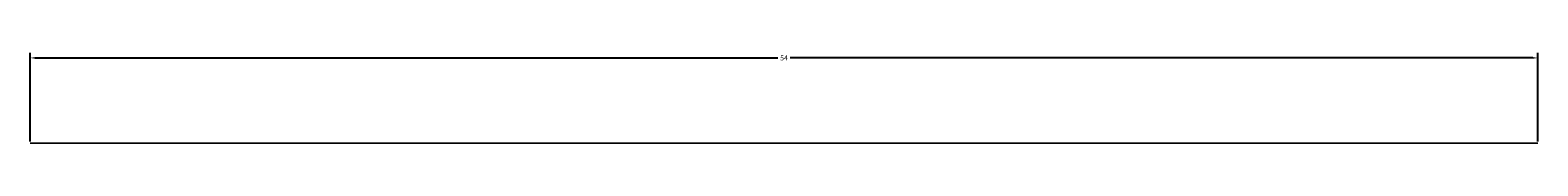
# Model space of a CAD drawing. Units: millimetres. Extents: x -5 to 2707, y 665 to 1247.
# Tile 2 of 3: x 2653 to 2707, y 665 to 668. Entities that reach past the tile are written whole.
import ezdxf

# ---------------------------------------------------------------- set-up
doc = ezdxf.new("R2010")
doc.units = ezdxf.units.MM
doc.layers.add('M-CONS', color=7, linetype='Continuous', lineweight=18)
doc.layers.add('M-DIMS', color=2, linetype='Continuous', lineweight=18)
doc.styles.get("Standard").update_dxf_attribs({"font": 'arial.ttf'})
doc.dimstyles.get("Standard").update_dxf_attribs({"dimtxt": 0.18, "dimasz": 0.18, "dimexe": 0.18, "dimexo": 0.0625, "dimgap": 0.09, "dimtad": 0, "dimtih": 1, "dimtoh": 1, "dimdec": 4, "dimzin": 0, "dimdsep": 46, "dimtxsty": 'Standard', "dimcen": 0.09, "dimadec": 0, "dimazin": 0, "dimtfac": 1, "dimtdec": 4, "dimtofl": 0, "dimtmove": 0, "dimatfit": 3, "dimfxl": 1, "dimtolj": 1, "dimtzin": 0, "dimarcsym": 0})

# ---------------------------------------------------------------- blocks, each defined once
blk = doc.blocks.new('*D15')
at = {"layer": 'Defpoints', "color": 0, "transparency": 16777216}
for p in [(2707.36, 668.157), (2653.36, 665.107), (2707.36, 665.107)]:
    blk.add_point(p, dxfattribs=at)
at = {"layer": 'M-DIMS', "color": 0, "lineweight": -2, "transparency": 16777216}
for p, q in [((2653.36, 665.169), (2653.36, 668.337)), ((2653.54, 668.157), (2680.141, 668.157)), ((2707.18, 668.157), (2680.578, 668.157)), ((2707.36, 665.169), (2707.36, 668.337))]:
    blk.add_line(p, q, dxfattribs=at)
at = {"layer": 'M-DIMS', "color": 0, "transparency": 16777216}
for points in [[(2653.54, 668.187), (2653.54, 668.127), (2653.36, 668.157)], [(2707.18, 668.187), (2707.18, 668.127), (2707.36, 668.157)]]:
    blk.add_solid(points, dxfattribs=at)
at = {"layer": 'M-DIMS', "color": 0, "transparency": 16777216, "insert": (2680.36, 668.157), "char_height": 0.18, "attachment_point": 5}
blk.add_mtext('\\A1;54', dxfattribs=at)

msp = doc.modelspace()

# ---------------------------------------------------------------- linework, layer by layer
at = {"layer": 'M-CONS', "extrusion": (0, -1, 0), "elevation": -665.1068}
msp.add_lwpolyline([(2668.3598, -3.4533), (2668.3598, 6.5467), (2653.3598, 6.5467), (2653.3598, -23.4533), (2707.3598, -23.4533), (2707.3598, 6.5467), (2692.3598, 6.5467), (2692.3598, -3.4533, -1)], format="xyb", close=True, dxfattribs=at)

# ---------------------------------------------------------------- dimensions: what is measured, and where the dimension line sits
at = {"layer": 'M-DIMS'}
dim = msp.add_linear_dim(base=(2707.3598, 668.1568), p1=(2653.3598, 665.1068), p2=(2707.3598, 665.1068), dimstyle='Standard', override={"dimdec": 0, "dimlfac": 1, "dimrnd": 0, "dimzin": 0, "dimdsep": 46, "dimlunit": 2}, dxfattribs=at)
dim.commit()
dim.dimension.update_dxf_attribs({"geometry": '*D15', "text_midpoint": (2680.3598, 668.1568)})

doc.saveas('drawing.dxf')
